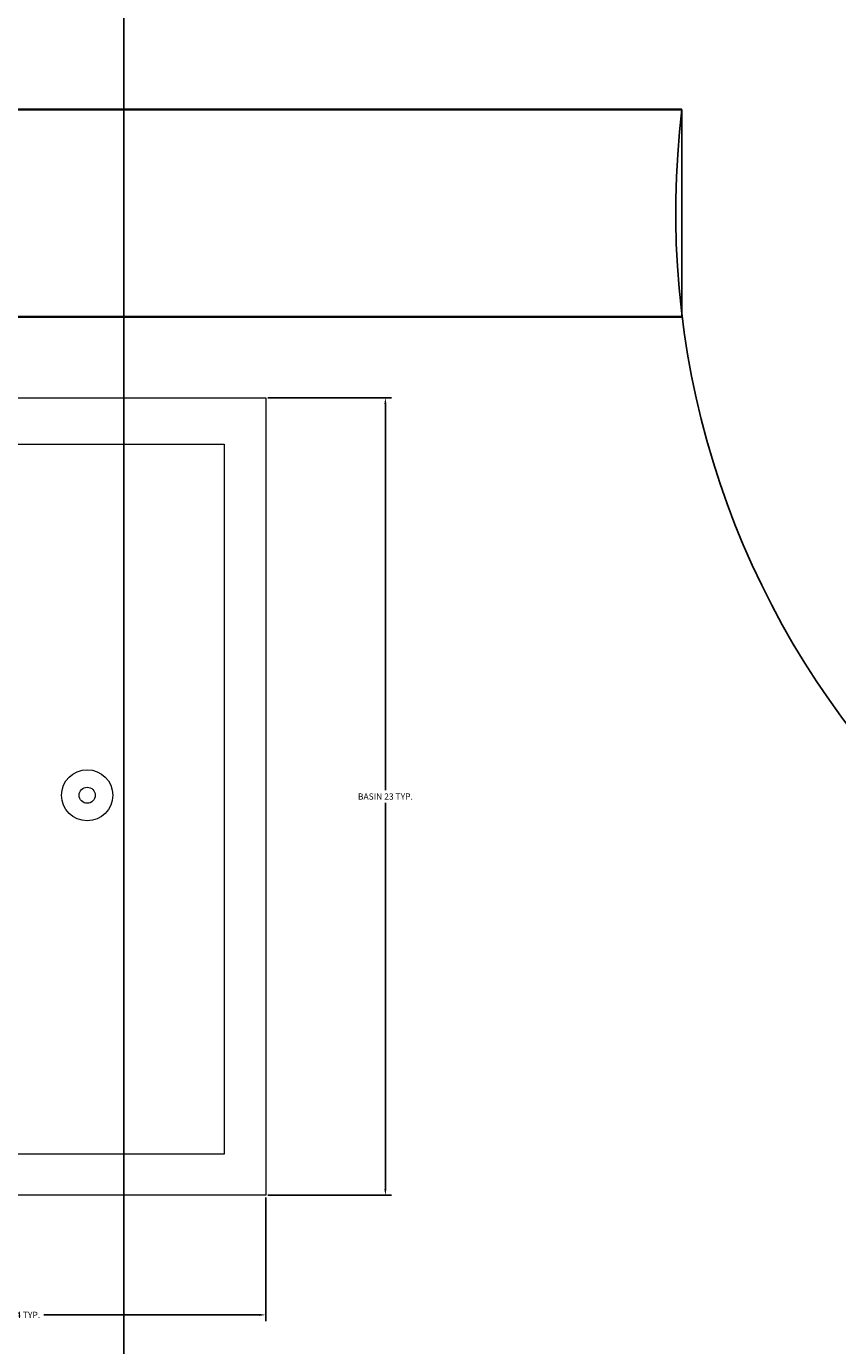
# Model space of a CAD drawing. Units: inches. Extents: x -61 to 1599, y -1316 to 257.
# Tile 88 of 204: x 274 to 298, y -318 to -280. Entities that reach past the tile are written whole.
import ezdxf

# ---------------------------------------------------------------- set-up
doc = ezdxf.new("R2010")
doc.units = ezdxf.units.IN
doc.header["$MEASUREMENT"] = 0
doc.linetypes.add('ACAD_ISO02W100', pattern=[15, 12, -3])
for name, color, linetype, lineweight in [('A-ANNO-DIMS', 2, 'Continuous', 18), ('A-FLOR-FIXT', 8, 'Continuous', 18), ('A-WALL-JAMB', 4, 'ACAD_ISO02W100', 25), ('DOORS', 2, 'Continuous', 25), ('WALLS', 4, 'Continuous', 35)]:
    doc.layers.add(name, color=color, linetype=linetype, lineweight=lineweight)
doc.styles.get("Standard").update_dxf_attribs({"font": 'arial.ttf'})
doc.dimstyles.get("Standard").update_dxf_attribs({"dimtxt": 0.18, "dimasz": 0.18, "dimexe": 0.18, "dimexo": 0.0625, "dimgap": 0.09, "dimtad": 0, "dimtih": 1, "dimtoh": 1, "dimdec": 0, "dimzin": 0, "dimdsep": 46, "dimlunit": 3, "dimtxsty": 'Standard', "dimcen": 0.09, "dimadec": 0, "dimazin": 0, "dimtfac": 1, "dimtdec": 0, "dimtofl": 0, "dimtmove": 0, "dimatfit": 3, "dimfxl": 1, "dimtolj": 1, "dimtzin": 0, "dimarcsym": 0})

# ---------------------------------------------------------------- blocks, each defined once
blk = doc.blocks.new('DOOR-SWING-24')
blk.add_line((0, 0), (0, 3.6))
blk.add_lwpolyline([(0, 0), (0, -24), (1.05, -24), (1.05, 0)], close=True)
blk.add_arc((-0.441, 0.618), 24.622, 271.0259, 6.9559)
blk = doc.blocks.new('LAVATORY-WALL-2')
blk.add_line((3.675, 10.958), (3.675, 12.185))
for points in [[(0, 23.069), (13.865, 23.069), (13.865, 0), (0, 0)], [(12.662, 21.727), (12.662, 1.185), (2.198, 1.185), (2.198, 21.727)], [(5.777, 12.185), (5.777, 10.958), (0.396, 10.958), (0.396, 12.185)]]:
    blk.add_lwpolyline(points, close=True)
for radius in [0.74, 0.233]:
    blk.add_circle((8.705, 11.571), radius)
blk.add_arc((-20.864, 11.456), 25.246, 335.9939, 24.0061)
blk = doc.blocks.new('*D626')
at = {"layer": 'A-ANNO-DIMS', "color": 0, "lineweight": -2, "transparency": 16777216}
for p, q in [((281.045, -290.661), (284.623, -290.661)), ((284.443, -290.841), (284.443, -302.012)), ((284.443, -313.55), (284.443, -302.379)), ((281.045, -313.73), (284.623, -313.73))]:
    blk.add_line(p, q, dxfattribs=at)
at = {"layer": 'A-ANNO-DIMS', "color": 0, "transparency": 16777216}
for points in [[(284.413, -290.841), (284.473, -290.841), (284.443, -290.661)], [(284.413, -313.55), (284.473, -313.55), (284.443, -313.73)]]:
    blk.add_solid(points, dxfattribs=at)
at = {"layer": 'DEFPOINTS', "color": 0, "transparency": 16777216}
for p in [(280.983, -290.661), (284.443, -290.661), (280.983, -313.73)]:
    blk.add_point(p, dxfattribs=at)
at = {"layer": 'A-ANNO-DIMS', "color": 0, "transparency": 16777216, "insert": (284.443, -302.195), "char_height": 0.18, "attachment_point": 5}
blk.add_mtext('\\A1;BASIN 23 TYP.', dxfattribs=at)
blk = doc.blocks.new('*D627')
at = {"layer": 'A-ANNO-DIMS', "color": 0, "lineweight": -2, "transparency": 16777216}
for p, q in [((267.117, -313.792), (267.117, -317.37)), ((280.983, -313.792), (280.983, -317.37)), ((267.297, -317.19), (273.53, -317.19)), ((280.803, -317.19), (274.569, -317.19))]:
    blk.add_line(p, q, dxfattribs=at)
at = {"layer": 'A-ANNO-DIMS', "color": 0, "transparency": 16777216}
for points in [[(267.297, -317.16), (267.297, -317.22), (267.117, -317.19)], [(280.803, -317.16), (280.803, -317.22), (280.983, -317.19)]]:
    blk.add_solid(points, dxfattribs=at)
at = {"layer": 'DEFPOINTS', "color": 0, "transparency": 16777216}
for p in [(267.117, -313.73), (280.983, -313.73), (280.983, -317.19)]:
    blk.add_point(p, dxfattribs=at)
at = {"layer": 'A-ANNO-DIMS', "color": 0, "transparency": 16777216, "insert": (274.05, -317.19), "char_height": 0.18, "attachment_point": 5}
blk.add_mtext('\\A1;14 TYP.', dxfattribs=at)
blk = doc.blocks.new('*D687')
at = {"layer": 'A-ANNO-DIMS', "color": 0, "lineweight": -2, "transparency": 16777216}
for p, q in [((289.418, 181.677), (-61.077, 181.677)), ((-60.897, 181.497), (-60.897, -528.952)), ((-60.897, -1239.765), (-60.897, -529.316)), ((319.64, -1239.945), (-61.077, -1239.945))]:
    blk.add_line(p, q, dxfattribs=at)
at = {"layer": 'A-ANNO-DIMS', "color": 0, "transparency": 16777216}
for points in [[(-60.927, 181.497), (-60.867, 181.497), (-60.897, 181.677)], [(-60.927, -1239.765), (-60.867, -1239.765), (-60.897, -1239.945)]]:
    blk.add_solid(points, dxfattribs=at)
at = {"layer": 'DEFPOINTS', "color": 0, "transparency": 16777216}
for p in [(289.481, 181.677), (-60.897, -1239.945), (319.703, -1239.945)]:
    blk.add_point(p, dxfattribs=at)
at = {"layer": 'A-ANNO-DIMS', "color": 0, "transparency": 16777216, "insert": (-60.897, -529.134), "char_height": 0.18, "attachment_point": 5}
blk.add_mtext('\\A1;1421.6', dxfattribs=at)
blk = doc.blocks.new('*D699')
at = {"layer": 'A-ANNO-DIMS', "color": 0, "lineweight": -2, "transparency": 16777216}
for p, q in [((835.64, -167.169), (-61.077, -167.169)), ((-60.897, -167.349), (-60.897, -306.726)), ((-60.897, -446.466), (-60.897, -307.09)), ((841.64, -446.646), (-61.077, -446.646))]:
    blk.add_line(p, q, dxfattribs=at)
at = {"layer": 'A-ANNO-DIMS', "color": 0, "transparency": 16777216}
for points in [[(-60.927, -167.349), (-60.867, -167.349), (-60.897, -167.169)], [(-60.927, -446.466), (-60.867, -446.466), (-60.897, -446.646)]]:
    blk.add_solid(points, dxfattribs=at)
at = {"layer": 'DEFPOINTS', "color": 0, "transparency": 16777216}
for p in [(835.703, -167.169), (-60.897, -446.646), (841.703, -446.646)]:
    blk.add_point(p, dxfattribs=at)
at = {"layer": 'A-ANNO-DIMS', "color": 0, "transparency": 16777216, "insert": (-60.897, -306.908), "char_height": 0.18, "attachment_point": 5}
blk.add_mtext('\\A1;279.5', dxfattribs=at)
blk = doc.blocks.new('*D702')
at = {"layer": 'A-ANNO-DIMS', "color": 0, "lineweight": -2, "transparency": 16777216}
for p, q in [((276.882, -616.882), (276.882, 257.457)), ((277.062, 257.277), (312.209, 257.277)), ((348.14, 257.277), (312.994, 257.277)), ((348.32, -616.882), (348.32, 257.457))]:
    blk.add_line(p, q, dxfattribs=at)
at = {"layer": 'A-ANNO-DIMS', "color": 0, "transparency": 16777216}
for points in [[(277.062, 257.307), (277.062, 257.247), (276.882, 257.277)], [(348.14, 257.307), (348.14, 257.247), (348.32, 257.277)]]:
    blk.add_solid(points, dxfattribs=at)
at = {"layer": 'DEFPOINTS', "color": 0, "transparency": 16777216}
for p in [(348.32, 257.277), (276.882, -616.945), (348.32, -616.945)]:
    blk.add_point(p, dxfattribs=at)
at = {"layer": 'A-ANNO-DIMS', "color": 0, "transparency": 16777216, "insert": (312.601, 257.277), "char_height": 0.18, "attachment_point": 5}
blk.add_mtext('\\A1;71.44', dxfattribs=at)

msp = doc.modelspace()

# ---------------------------------------------------------------- linework, layer by layer
at = {"layer": 'A-WALL-JAMB'}
msp.add_line((293.017, -282.3229), (293.017, -288.3229), dxfattribs=at)
at = {"layer": 'WALLS'}
for p, q in [((258.999, -282.3229), (293.017, -282.3229)), ((265.7028, -288.3229), (293.0214, -288.3229))]:
    msp.add_line(p, q, dxfattribs=at)

# ---------------------------------------------------------------- block references
at = {"layer": 'A-FLOR-FIXT'}
msp.add_blockref('LAVATORY-WALL-2', (267.1172, -313.7295), dxfattribs=at)
at = {"layer": 'DOORS', "extrusion": (0, 0, -1), "zscale": -1}
msp.add_blockref('DOOR-SWING-24', (-317.017, -285.9229), dxfattribs=at)

# ---------------------------------------------------------------- dimensions: what is measured, and where the dimension line sits
at = {"layer": 'A-ANNO-DIMS'}
dim = msp.add_linear_dim(base=(348.3201, 257.2771), p1=(276.8825, -616.9446), p2=(348.3201, -616.9446), dimstyle='Standard', override={"dimdec": 2, "dimlfac": 1, "dimrnd": 0, "dimzin": 0, "dimdsep": 46, "dimlunit": 2}, dxfattribs=at)
dim.commit()
dim.dimension.update_dxf_attribs({"geometry": '*D702', "text_midpoint": (312.6013, 257.2771)})
for base, p1, p2, picture, middle in [((-60.8972, -1239.9446), (289.4807, 181.6771), (319.7028, -1239.9446), '*D687', (-60.8972, -529.1337)), ((-60.8972, -446.6462), (835.7028, -167.169), (841.7028, -446.6462), '*D699', (-60.8972, -306.9076))]:
    dim = msp.add_linear_dim(base=base, p1=p1, p2=p2, angle=90, dimstyle='Standard', override={"dimdec": 1, "dimlfac": 1, "dimrnd": 0, "dimzin": 0, "dimdsep": 46, "dimlunit": 2}, dxfattribs=at)
    dim.commit()
    dim.dimension.update_dxf_attribs({"geometry": picture, "text_midpoint": middle})
dim = msp.add_linear_dim(base=(284.443, -290.6609), p1=(280.9827, -313.73), p2=(280.9827, -290.6609), angle=90, text='BASIN <> TYP.', dimstyle='Standard', override={"dimdec": 0, "dimlfac": 1, "dimrnd": 0, "dimzin": 0, "dimdsep": 46, "dimlunit": 2}, dxfattribs=at)
dim.commit()
dim.dimension.update_dxf_attribs({"geometry": '*D626', "text_midpoint": (284.443, -302.1955)})
dim = msp.add_linear_dim(base=(280.9827, -317.1903), p1=(267.117, -313.73), p2=(280.9827, -313.73), text='<> TYP.', dimstyle='Standard', override={"dimdec": 0, "dimlfac": 1, "dimrnd": 0, "dimzin": 0, "dimdsep": 46, "dimlunit": 2}, dxfattribs=at)
dim.commit()
dim.dimension.update_dxf_attribs({"geometry": '*D627', "text_midpoint": (274.0498, -317.1903)})

doc.saveas('drawing.dxf')
